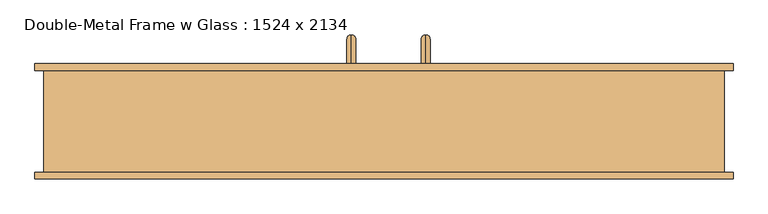
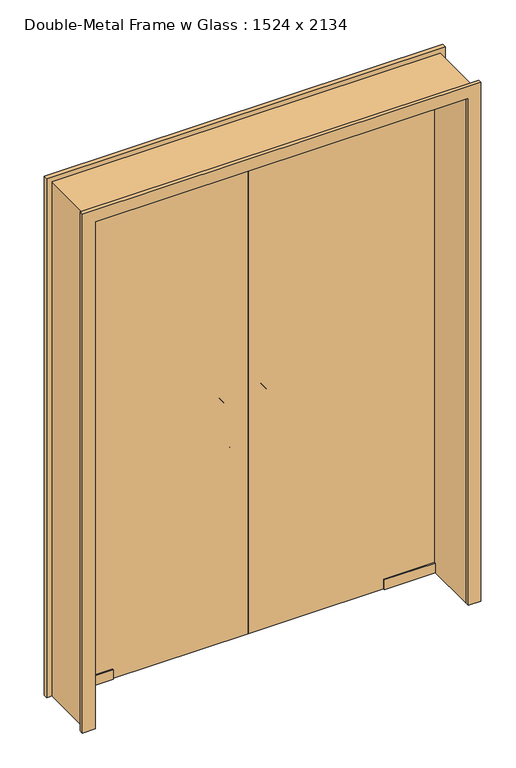
"""IFC4 building model written with IfcOpenShell, lengths in millimetres: door geometry, Double-Metal Frame w Glass : 1524 x 2134."""

from ifc_helpers import new_model, si_unit, frame, origin, origin_with_axes, place, context, project, spatial, polyline, circle_curve, ellipse_curve, outline, extrude, source, transform, mapped, element, save
from ifc_brep_helpers import plane_surface, cylinder_surface, advanced_brep


def double_metal_frame_w_glass_1524_x_2134_5eb37b3f(model_context):
    return source(origin(), model_context, "Body", "SolidModel", [
        extrude(outline(polyline([(532.0, 94.3), (732.0, 94.3), (732.0, 74.1257896), (532.0, 74.1257896), (532.0, 94.3)])), origin_with_axes(), (0.0, 0.0, 1.0), 40.0),
        extrude(outline(polyline([(532.0, 94.3), (732.0, 94.3), (732.0, 74.1257896), (532.0, 74.1257896), (532.0, 94.3)])), frame((0.0, 0.0, 2063.6), z_axis=(0.0, 0.0, 1.0), x_axis=(1.0, 0.0, 0.0)), (0.0, 0.0, 1.0), 40.0),
        extrude(outline(polyline([(-732.0, 94.3), (-532.0, 94.3), (-532.0, 74.1620837), (-732.0, 74.1620837), (-732.0, 94.3)])), frame((0.0, 0.0, 2063.6), z_axis=(0.0, 0.0, 1.0), x_axis=(1.0, 0.0, 0.0)), (0.0, 0.0, 1.0), 40.0),
        extrude(outline(polyline([(-732.0, 94.3), (-532.0, 94.3), (-532.0, 74.1620837), (-732.0, 74.1620837), (-732.0, 94.3)])), origin_with_axes(), (0.0, 0.0, 1.0), 40.0),
        advanced_brep(
        [(-73.3333333, 89.3, 935.0), (-73.3333333, 89.3, 955.0), (-73.3333333, 154.3, 935.0), (-73.3333333, 174.3, 955.0), (-73.3333333, 154.3, 795.0), (-73.3333333, 174.3, 775.0), (-73.3333333, 89.3, 795.0), (-73.3333333, 89.3, 775.0)],
        [
            (0, 1, circle_curve(frame((-73.3333333, 89.3, 945.0), z_axis=(0.0, -1.0, 0.0), x_axis=(0.0, 0.0, 1.0)), 10.0)),
            (1, 0, circle_curve(frame((-73.3333333, 89.3, 945.0), z_axis=(0.0, -1.0, 0.0), x_axis=(0.0, 0.0, 1.0)), 10.0)),
            (0, 2),
            (2, 3, ellipse_curve(frame((-73.3333333, 164.3, 945.0), z_axis=(0.0, -0.7071067811865475, 0.7071067811865475), x_axis=(0.0, -0.7071067811865476, -0.7071067811865474)), 14.1421356, 10.0)),
            (3, 1),
            (3, 2, ellipse_curve(frame((-73.3333333, 164.3, 945.0), z_axis=(0.0, -0.7071067811865475, 0.7071067811865475), x_axis=(0.0, -0.7071067811865476, -0.7071067811865474)), 14.1421356, 10.0)),
            (2, 4),
            (4, 5, ellipse_curve(frame((-73.3333333, 164.3, 785.0), z_axis=(0.0, 0.7071067811865475, 0.7071067811865475), x_axis=(0.0, -0.7071067811865474, 0.7071067811865476)), 14.1421356, 10.0)),
            (5, 3),
            (5, 4, ellipse_curve(frame((-73.3333333, 164.3, 785.0), z_axis=(0.0, 0.7071067811865475, 0.7071067811865475), x_axis=(0.0, -0.7071067811865474, 0.7071067811865476)), 14.1421356, 10.0)),
            (6, 7, circle_curve(frame((-73.3333333, 89.3, 785.0), z_axis=(0.0, -1.0, 0.0), x_axis=(0.0, 0.0, -1.0)), 10.0)),
            (7, 6, circle_curve(frame((-73.3333333, 89.3, 785.0), z_axis=(0.0, -1.0, 0.0), x_axis=(0.0, 0.0, -1.0)), 10.0)),
            (4, 6),
            (7, 5),
        ],
        [
            plane_surface(frame((-102.2533066, 89.3, 945.0), z_axis=(0.0, -1.0, 0.0), x_axis=(0.0, 0.0, 1.0))),
            cylinder_surface(frame((-73.3333333, 89.3, 945.0), z_axis=(0.0, -1.0, 0.0), x_axis=(0.0, 0.0, 1.0)), 10.0),
            cylinder_surface(frame((-73.3333333, 164.3, 945.0), z_axis=(0.0, 0.0, 1.0), x_axis=(0.0, 1.0, 0.0)), 10.0),
            plane_surface(frame((-102.2533066, 89.3, 785.0), z_axis=(0.0, -1.0, 0.0), x_axis=(0.0, 0.0, -1.0))),
            cylinder_surface(frame((-73.3333333, 164.3, 785.0), z_axis=(0.0, 1.0, 0.0), x_axis=(0.0, 0.0, -1.0)), 10.0),
        ],
        [
            (0, [[1, 2]]),
            (1, [[-1, 3, 4, 5]]),
            (1, [[-2, -5, 6, -3]]),
            (2, [[-4, 7, 8, 9]]),
            (2, [[-6, -9, 10, -7]]),
            (3, [[11, 12]]),
            (4, [[-8, 13, -12, 14]]),
            (4, [[-10, -14, -11, -13]]),
        ],
    ),
        advanced_brep(
        [(93.4707339, 89.3, 935.0), (93.4707339, 89.3, 955.0), (93.4707339, 154.3, 935.0), (93.4707339, 174.3, 955.0), (93.4707339, 154.3, 795.0), (93.4707339, 174.3, 775.0), (93.4707339, 89.3, 795.0), (93.4707339, 89.3, 775.0)],
        [
            (0, 1, circle_curve(frame((93.4707339, 89.3, 945.0), z_axis=(0.0, -1.0, 0.0), x_axis=(0.0, 0.0, 1.0)), 10.0)),
            (1, 0, circle_curve(frame((93.4707339, 89.3, 945.0), z_axis=(0.0, -1.0, 0.0), x_axis=(0.0, 0.0, 1.0)), 10.0)),
            (0, 2),
            (2, 3, ellipse_curve(frame((93.4707339, 164.3, 945.0), z_axis=(0.0, -0.7071067811865475, 0.7071067811865475), x_axis=(0.0, -0.7071067811865476, -0.7071067811865474)), 14.1421356, 10.0)),
            (3, 1),
            (3, 2, ellipse_curve(frame((93.4707339, 164.3, 945.0), z_axis=(0.0, -0.7071067811865475, 0.7071067811865475), x_axis=(0.0, -0.7071067811865476, -0.7071067811865474)), 14.1421356, 10.0)),
            (2, 4),
            (4, 5, ellipse_curve(frame((93.4707339, 164.3, 785.0), z_axis=(0.0, 0.7071067811865475, 0.7071067811865475), x_axis=(0.0, -0.7071067811865474, 0.7071067811865476)), 14.1421356, 10.0)),
            (5, 3),
            (5, 4, ellipse_curve(frame((93.4707339, 164.3, 785.0), z_axis=(0.0, 0.7071067811865475, 0.7071067811865475), x_axis=(0.0, -0.7071067811865474, 0.7071067811865476)), 14.1421356, 10.0)),
            (6, 7, circle_curve(frame((93.4707339, 89.3, 785.0), z_axis=(0.0, -1.0, 0.0), x_axis=(0.0, 0.0, -1.0)), 10.0)),
            (7, 6, circle_curve(frame((93.4707339, 89.3, 785.0), z_axis=(0.0, -1.0, 0.0), x_axis=(0.0, 0.0, -1.0)), 10.0)),
            (4, 6),
            (7, 5),
        ],
        [
            plane_surface(frame((-102.2533066, 89.3, 945.0), z_axis=(0.0, -1.0, 0.0), x_axis=(0.0, 0.0, 1.0))),
            cylinder_surface(frame((93.4707339, 89.3, 945.0), z_axis=(0.0, -1.0, 0.0), x_axis=(0.0, 0.0, 1.0)), 10.0),
            cylinder_surface(frame((93.4707339, 164.3, 945.0), z_axis=(0.0, 0.0, 1.0), x_axis=(0.0, 1.0, 0.0)), 10.0),
            plane_surface(frame((-102.2533066, 89.3, 785.0), z_axis=(0.0, -1.0, 0.0), x_axis=(0.0, 0.0, -1.0))),
            cylinder_surface(frame((93.4707339, 164.3, 785.0), z_axis=(0.0, 1.0, 0.0), x_axis=(0.0, 0.0, -1.0)), 10.0),
        ],
        [
            (0, [[1, 2]]),
            (1, [[-1, 3, 4, 5]]),
            (1, [[-2, -5, 6, -3]]),
            (2, [[-4, 7, 8, 9]]),
            (2, [[-6, -9, 10, -7]]),
            (3, [[11, 12]]),
            (4, [[-8, 13, -12, 14]]),
            (4, [[-10, -14, -11, -13]]),
        ],
    ),
        extrude(outline(polyline([(-732.0, 89.6031221), (0.0, 89.6031221), (0.0, 79.3), (-732.0, 79.3), (-732.0, 89.6031221)])), origin_with_axes(), (0.0, 0.0, 1.0), 2103.6),
        extrude(outline(polyline([(0.0, 89.3), (732.0, 89.3), (732.0, 79.3), (0.0, 79.3), (0.0, 89.3)])), origin_with_axes(), (0.0, 0.0, 1.0), 2103.6),
        extrude(outline(polyline([(0.0, 732.0), (0.0, 782.0), (2153.6, 782.0), (2153.6, -782.0), (0.0, -782.0), (0.0, -732.0), (2103.6, -732.0), (2103.6, 732.0), (0.0, 732.0)])), frame((0.0, 94.3, 0.0), z_axis=(0.0, 1.0, 0.0), x_axis=(0.0, 0.0, 1.0)), (0.0, 0.0, 1.0), 15.0),
        extrude(outline(polyline([(0.0, -782.0), (0.0, -732.0), (2103.6, -732.0), (2103.6, 732.0), (0.0, 732.0), (0.0, 782.0), (2153.6, 782.0), (2153.6, -782.0), (0.0, -782.0)])), frame((0.0, -149.1984743, 0.0), z_axis=(0.0, 1.0, 0.0), x_axis=(0.0, 0.0, 1.0)), (0.0, 0.0, 1.0), 14.8984743),
        extrude(outline(polyline([(0.0, 732.0), (0.0, 762.0), (2133.6, 762.0), (2133.6, -762.0), (0.0, -762.0), (0.0, -732.0), (2103.6, -732.0), (2103.6, 732.0), (0.0, 732.0)])), frame((0.0, -134.3, 0.0), z_axis=(0.0, 1.0, 0.0), x_axis=(0.0, 0.0, 1.0)), (0.0, 0.0, 1.0), 228.6),
    ])


if __name__ == "__main__":
    model = new_model("IFC4")
    model_context = context("Model", 3, world=origin())
    ifc_project = project(units=[si_unit("LENGTHUNIT", "METRE", prefix="MILLI")], contexts=[model_context])
    site = spatial("IfcSite", under=ifc_project)
    building = spatial("IfcBuilding", under=site)
    placement = place(None, origin())
    double_metal_frame_w_glass_1524_x_2134_shape = double_metal_frame_w_glass_1524_x_2134_5eb37b3f(model_context)
    element("IfcDoor", 1, ObjectType="Double-Metal Frame w Glass : 1524 x 2134", at=placement, inside=building, context=model_context, shape_type="MappedRepresentation", body=[
        mapped(double_metal_frame_w_glass_1524_x_2134_shape, transform((0.0, 0.0, 0.0), x_axis=(1.0, 0.0, 0.0), y_axis=(0.0, 1.0, 0.0), z_axis=(0.0, 0.0, 1.0))),
    ])
    save(model, "model.ifc")

# Revit data of these elements
# Type "Double-Metal Frame w Glass : 1524 x 2134"
#   Type Mark = "17"
#   Operation = "DoubleDoorSingleSwing"
#   Keynote = "L20"
#   Analytic Construction = "<None>"
#   Height = 7' - 0"
#   Width = 5' - 0"
#   Define Thermal Properties by = 1
#   Wall Closure = (empty or 0)
#   Function = (empty or 0)
# Element 1 (IfcDoor, "Double-Metal Frame w Glass : 1524 x 2134")
#   Materials on its faces: "Chrome", "Default Metal Frame", "Glass"
# Materials
#   "Chrome": colour RGB 192 192 192, transparency 0
#   "Default Metal Frame": colour RGB 132 153 165, transparency 0
#   "Glass": class "Glass", colour RGB 0 128 192, transparency 0.75, Description = "Soda Lime Glass", Cost = 0
